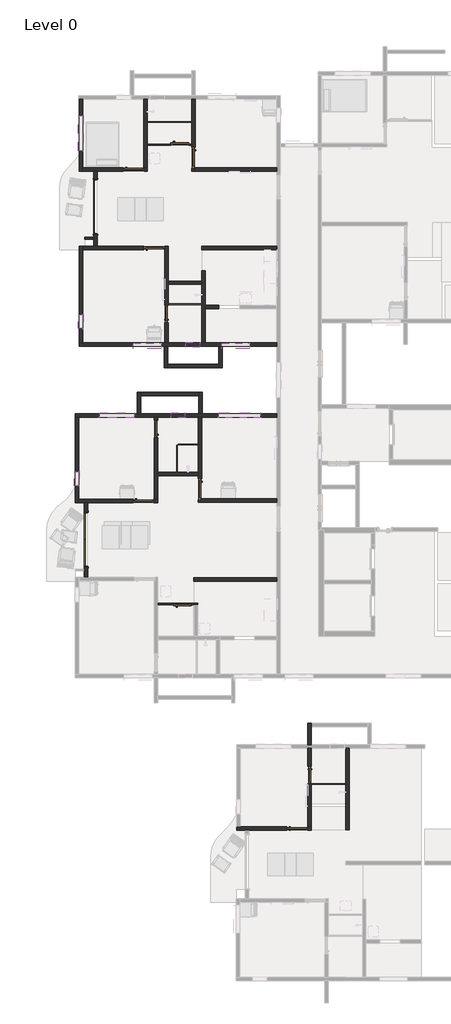
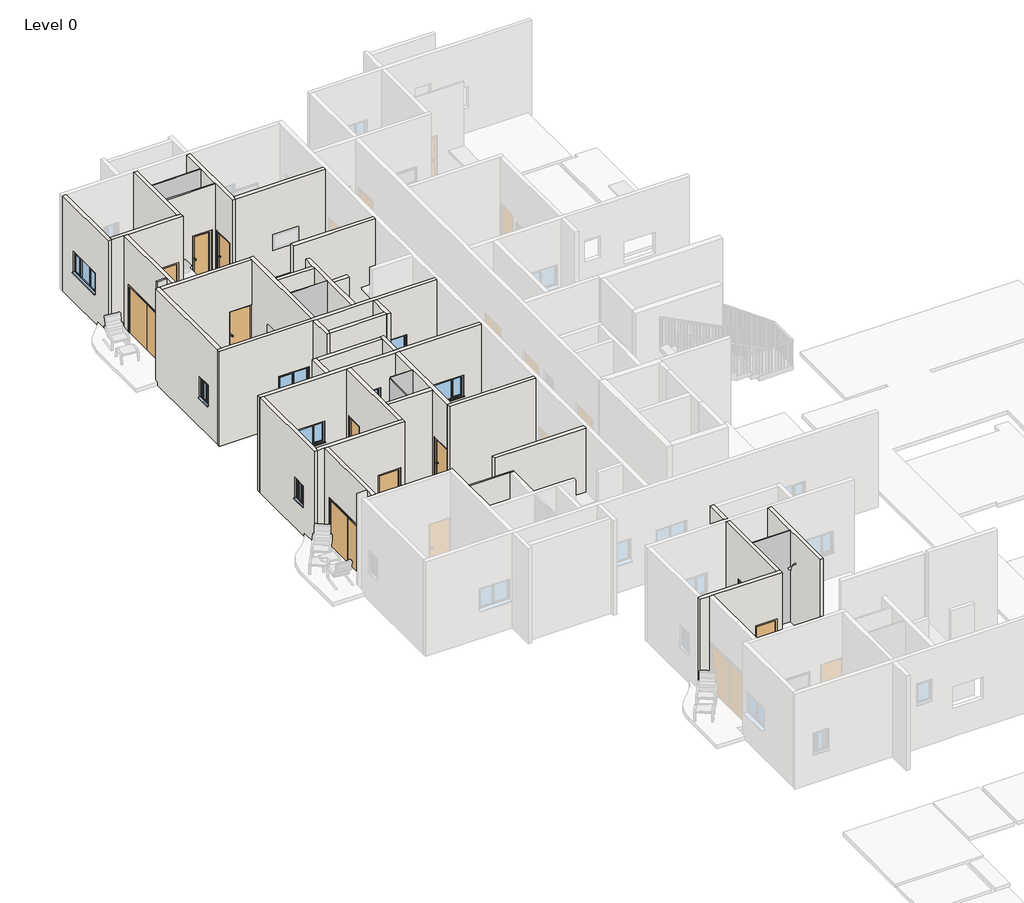
# One storey, part 4 of 14: 35 walls, 14 doors, 9 windows, 5 plates.
# Revit data of these elements (continued)
# Type "Windows_Tpl_Variable_Casement : 5'" (continued)
#   Cill Depth = 87.5 mm
#   Cavity Closer Width = 50 mm
#   Cavity Closer Offset from Ext = 102.5 mm
#   Cavity Closer Depth = 85 mm
#   Casement Width = 450 mm
#   Vis - Cavity Closers = yes
#   Define Thermal Properties by = 1
#   Material Trim = Window Frame
#   Material Glass = Glass
#   Material Frame = Window Frame
#   Wall Closure = (empty or 0)
# Type "Windows_Tpl_Variable_Casement : 6'"
#   Type Mark = "84"
#   Operation = "TriplePanelVertical"
#   Construction Type Id = "GSP4R"
#   Manufacturer = "Revit"
#   Keynote = "L10"
#   Analytic Construction = "1/8 in Pilkington single glazing"
#   Wrap Layers (Int) from Ext = 177.5 mm
#   Wrap Layers (Ext) from Ext = 102.5 mm
#   Window Board Projection = 25 mm
#   Window Board Extension = 25 mm
#   Visual Light Transmittance = 0.9
#   Solar Heat Gain Coefficient = 0.78
#   Rough Width = 1828.8 mm
#   Rough Height = 910 mm
#   Height = 910 mm
#   Width = 1828.8 mm
#   Heat Transfer Coefficient (U) = 3.6886 W/(m²·K)
#   Glazing Thickness = 24 mm
#   FrameOffset - External = 50 mm
#   Frame Depth = 65 mm
#   Default Head Height = 2110 mm
#   Cill Depth = 87.5 mm
#   Cavity Closer Width = 50 mm
#   Cavity Closer Offset from Ext = 102.5 mm
#   Cavity Closer Depth = 85 mm
#   Casement Width = 450 mm
#   Vis - Cavity Closers = yes
#   Define Thermal Properties by = 1
#   Material Trim = Window Frame
#   Material Glass = Glass
#   Material Frame = Window Frame
#   Wall Closure = (empty or 0)
# Elements 1, 2 (IfcDoor, "Doors_Concept_IntDbl : 8'")
#   Phase Created = New Construction
#   Materials on its faces: "Glass", "Glass, Clear Glazing"
# Elements 3, 4, 5, 6, 7, 8 (IfcDoor, "Doors_ExtSgl_Flush : D2")
#   Phase Created = New Construction
#   Materials on its faces: "Door - Handle", "Door - Frame/Mullion", "Door - Panel"
# Elements 9, 10, 11, 12, 13, 14 (IfcDoor, "Doors_ExtSgl_Flush : D3")
#   Phase Created = New Construction
#   Materials on its faces: "Door - Handle", "Door - Frame/Mullion", "Door - Panel"
# Elements 15, 16, 17, 18, 19 (IfcPlate, "System Panel : Glazed")
#   Phase Created = New Construction
#   Materials on its faces: "Glass"
# Elements 20, 21, 22, 23, 24, 25, 26, 27, 28, 29, 30, 31, 32, 33, 34, 35, 36, 37, 38, 39, 40, 41, 42, 43, 44, 45, 46, 47, 48, 49, 50, 51 (IfcWall, "W1")
#   Top Offset = 0 mm
#   Base Offset = 0 mm
#   wall height = 4000 mm
#   Phase Created = New Construction
#   Base Constraint = Level 0
#   Top Constraint = Level 1
#   Materials on its faces: "Brick, Common"
# Element 52 (IfcWall, "W2")
#   Top Offset = 0 mm
#   Base Offset = 0 mm
#   wall height = 4000 mm
#   Phase Created = New Construction
#   Base Constraint = Level 0
#   Top Constraint = Level 1
#   Materials on its faces: "Brick, Common"
# Elements 53, 54 (IfcWall, "W4")
#   Top Offset = 0 mm
#   Base Offset = 0 mm
#   wall height = 4000 mm
#   Phase Created = New Construction
#   Base Constraint = Level 0
#   Top Constraint = Level 1
#   Materials on its faces: "Brick, Common"
# Element 55 (IfcWindow, "Windows_Concept_Plain_Dbl : 4'")
#   Mark = "46"
#   Phase Created = New Construction
#   Materials on its faces: "Window Frame", "Glass"
# Element 56 (IfcWindow, "Windows_Concept_Plain_Dbl : 4'")
#   Mark = "47"
#   Phase Created = New Construction
#   Materials on its faces: "Window Frame", "Glass"
# Element 57 (IfcWindow, "Windows_Sgl_Plain : 2'")
#   Mark = "50"
#   Phase Created = New Construction
#   Materials on its faces: "Window Frame", "Glass"
# Element 58 (IfcWindow, "Windows_Sgl_Plain : 2'")
#   Mark = "58"
#   Phase Created = New Construction
#   Materials on its faces: "Window Frame", "Glass"
# Element 59 (IfcWindow, "Windows_Tpl_Variable_Casement : 2'")
#   Mark = "48"
#   Phase Created = New Construction
#   Materials on its faces: "Window Frame", "Glass"
# Element 60 (IfcWindow, "Windows_Tpl_Variable_Casement : 2'")
#   Mark = "52"
#   Phase Created = New Construction
#   Materials on its faces: "Window Frame", "Glass"
# Element 61 (IfcWindow, "Windows_Tpl_Variable_Casement : 5'")
#   Mark = "45"
#   Phase Created = New Construction
#   Materials on its faces: "Window Frame", "Glass"
# Element 62 (IfcWindow, "Windows_Tpl_Variable_Casement : 5'")
#   Mark = "51"
#   Phase Created = New Construction
#   Materials on its faces: "Window Frame", "Glass"
# Element 63 (IfcWindow, "Windows_Tpl_Variable_Casement : 6'")
#   Mark = "53"
#   Phase Created = New Construction
#   Materials on its faces: "Window Frame", "Glass"
# Materials
#   "Glass": class "Glass", colour RGB 0 128 192, transparency 0.9, Description = "Soda Lime Glass", Cost = 0
#   "Glass, Clear Glazing": class "Glass", colour RGB 0 128 192, transparency 0.75, Description = "Clear glazing", Cost = 0
#   "Door - Panel": class "Wood", colour RGB 210 159 95, transparency 0, Keynote = "L20", Cost = 0
#   "Door - Frame/Mullion": class "Wood", colour RGB 212 179 113, transparency 0, Keynote = "L20", Cost = 0
#   "Door - Handle": colour RGB 0 0 0, transparency 0, Keynote = "P21", Cost = 0
#   "Brick, Common": class "Masonry", colour RGB 170 100 105, transparency 0, Description = "Common brick", Cost = 0
#   "Window Frame": colour RGB 249 249 249, transparency 0, Keynote = "L10", Cost = 0
